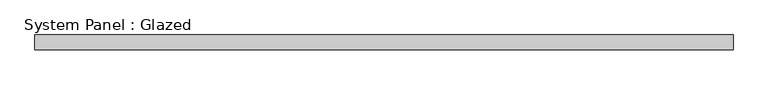
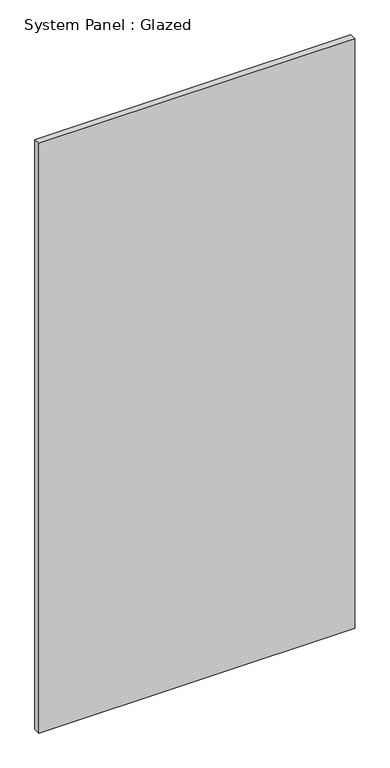
"""IFC4 building model written with IfcOpenShell, lengths in millimetres: plate geometry, System Panel : Glazed."""

from ifc_helpers import new_model, si_unit, origin, origin_with_axes, place, context, project, spatial, polyline, outline, extrude, source, transform, mapped, element, save


def system_panel_glazed_d0e49211(model_context):
    return source(origin(), model_context, "Body", "SweptSolid", [
        extrude(outline(polyline([(593.7250001, -44.45), (-593.7250001, -44.45), (-593.7250001, -19.05), (593.7250001, -19.05), (593.7250001, -44.45)])), origin_with_axes(), (0.0, 0.0, 1.0), 2343.15),
    ])


if __name__ == "__main__":
    model = new_model("IFC4")
    model_context = context("Model", 3, world=origin())
    ifc_project = project(units=[si_unit("LENGTHUNIT", "METRE", prefix="MILLI")], contexts=[model_context])
    site = spatial("IfcSite", under=ifc_project)
    building = spatial("IfcBuilding", under=site)
    placement = place(None, origin())
    system_panel_glazed_shape = system_panel_glazed_d0e49211(model_context)
    element("IfcPlate", 1, ObjectType="System Panel : Glazed", at=placement, inside=building, context=model_context, shape_type="MappedRepresentation", body=[
        mapped(system_panel_glazed_shape, transform((0.0, 0.0, 0.0), x_axis=(1.0, 0.0, 0.0), y_axis=(0.0, 1.0, 0.0), z_axis=(0.0, 0.0, 1.0))),
    ])
    save(model, "model.ifc")

# Revit data of these elements
# Type "System Panel : Glazed"
#   Construction Type Id = "GSP4R"
#   Analytic Construction = "1/8 in Pilkington single glazing"
#   Visual Light Transmittance = 0.9
#   Solar Heat Gain Coefficient = 0.86
#   Heat Transfer Coefficient (U) = 1.18115 BTU/(h·ft²·°F)
#   Define Thermal Properties by = 1
# Element 1 (IfcPlate, "System Panel : Glazed")
#   Materials on its faces: "glass panel 223"
# Materials
#   "glass panel 223": class "Generic", colour RGB 120 120 120, transparency 0, Cost = 0
